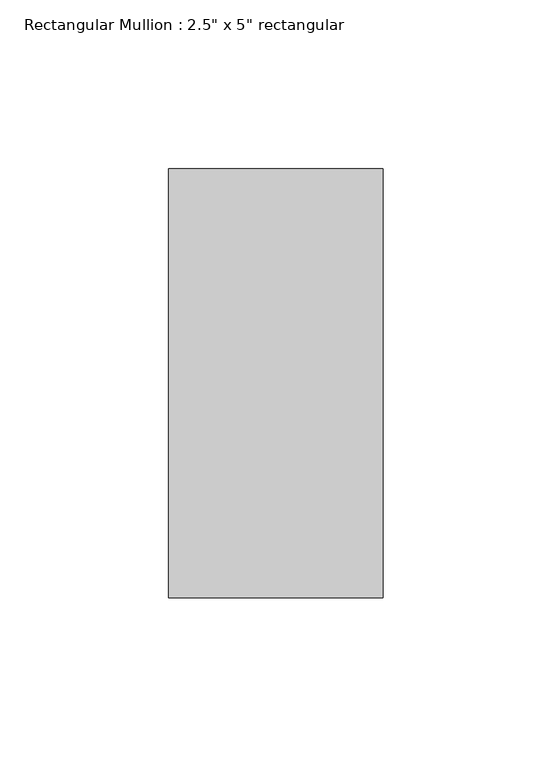
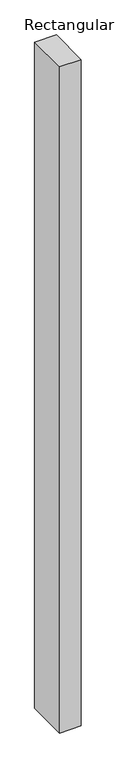
"""IFC4 building model written with IfcOpenShell, lengths in millimetres: member geometry."""

from ifc_helpers import new_model, si_unit, frame, origin, place, context, project, spatial, polyline, outline, extrude, source, transform, mapped, element, save


def member_760f9554(model_context):
    return source(origin(), model_context, "Body", "SweptSolid", [
        extrude(outline(polyline([(0.0, 63.5), (0.0, -63.5), (-63.5, -63.5), (-63.5, 63.5), (0.0, 63.5)])), frame((0.0, 0.0, -2070.1), z_axis=(0.0, 0.0, 1.0), x_axis=(1.0, 0.0, 0.0)), (0.0, 0.0, 1.0), 2070.1),
    ])


if __name__ == "__main__":
    model = new_model("IFC4")
    model_context = context("Model", 3, world=origin())
    ifc_project = project(units=[si_unit("LENGTHUNIT", "METRE", prefix="MILLI")], contexts=[model_context])
    site = spatial("IfcSite", under=ifc_project)
    building = spatial("IfcBuilding", under=site)
    placement = place(None, origin())
    member_shape = member_760f9554(model_context)
    element("IfcMember", 1, ObjectType="Rectangular Mullion : 2.5\" x 5\" rectangular", at=placement, inside=building, context=model_context, shape_type="MappedRepresentation", body=[
        mapped(member_shape, transform((0.0, 0.0, 0.0), x_axis=(1.0, 0.0, 0.0), y_axis=(0.0, 1.0, 0.0), z_axis=(0.0, 0.0, 1.0))),
    ])
    save(model, "model.ifc")

# Revit data of these elements
# Type "Rectangular Mullion : 2.5\" x 5\" rectangular"
#   built-in parameter 1007304 = 0.416667 (stored number, unit not read)
#   built-in parameter 1007301 = 0.104167 (stored number, unit not read)
#   built-in parameter 1007300 = 0.104167 (stored number, unit not read)
# Element 1 (IfcMember, "Rectangular Mullion : 2.5\" x 5\" rectangular")
#   Materials on its faces: "Aluminum"
# Materials
#   "Aluminum": class "Metal", colour RGB 247 247 247, transparency 0, Description = "Aluminum 6061", Cost = 0
